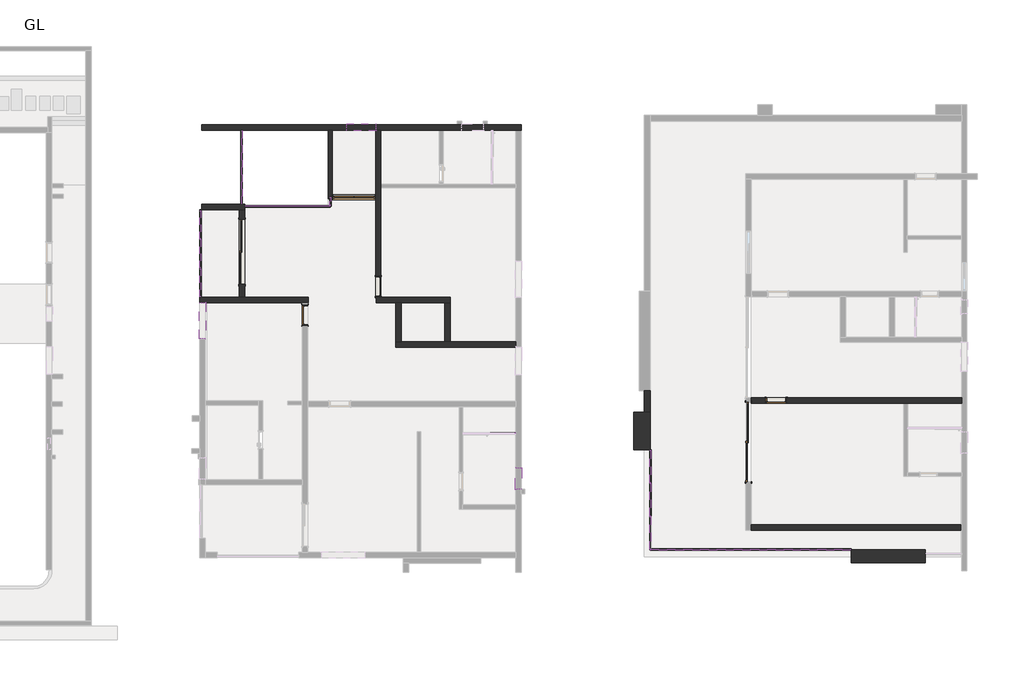
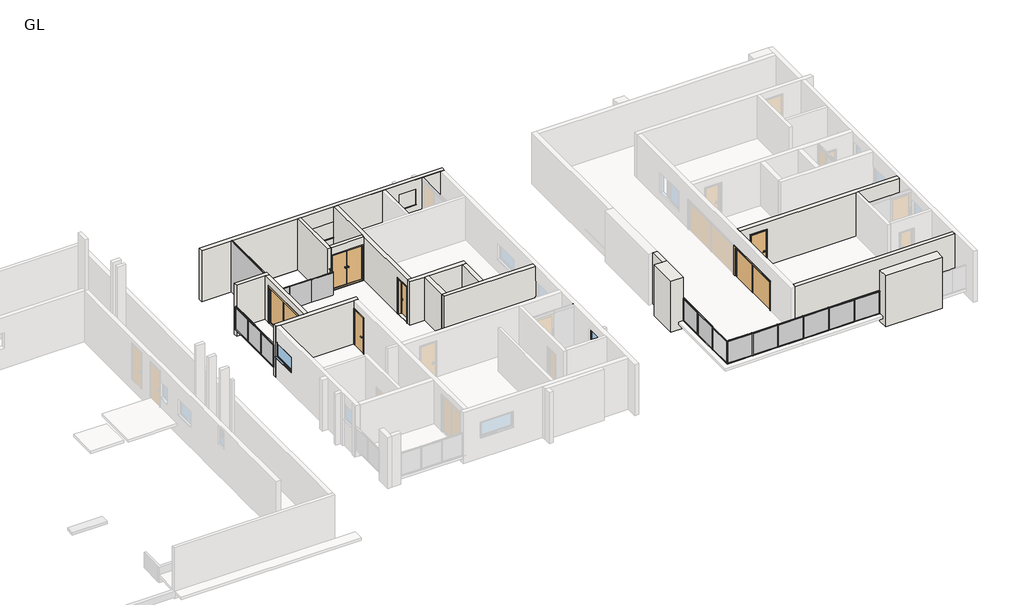
# One storey, part 3 of 6: 60 members, 17 walls, 16 plates, 6 doors, 3 windows.
"""IFC4 building model written with IfcOpenShell, lengths in millimetres."""

from ifc_helpers import new_model, si_unit, frame, origin, origin_with_axes, place, context, project, spatial, polyline, outline, extrude, faceted_brep, transform, mapped, element, save
from components import door_11_423d414f, door_9_db2a89ef, doors_extdbl_flush_1810x2110mm_0705243e, door_61435f0d, rectangular_mullion_30mm_square_7ad516a4, rectangular_mullion_30mm_square_4b249e81, rectangular_mullion_30mm_square_cc57b060, rectangular_mullion_30mm_square_bfb5791d, rectangular_mullion_30mm_square_48e0410f, rectangular_mullion_30mm_square_a54bfe06, rectangular_mullion_30mm_square_817e3251, rectangular_mullion_30mm_square_75078aee, rectangular_mullion_30mm_square_ea944ed7, rectangular_mullion_30mm_square_eb1e678b, rectangular_mullion_30mm_square_4b8855c0, rectangular_mullion_30mm_square_0acd70fe, rectangular_mullion_30mm_square_cec16e38, rectangular_mullion_30mm_square_28ebc8b3, rectangular_mullion_30mm_square_b4ecd99e, rectangular_mullion_30mm_square_04db908b, system_panel_glazed_bb4db1d5, system_panel_glazed_b6747f4f, system_panel_glazed_7e3392a4, system_panel_glazed_b055ca82, system_panel_glazed_df7e0718, system_panel_glazed_e520f566, windows_sgl_plain_3_28d0678b, windows_sgl_plain_4_aaf4c78a, windows_sgl_plain_5_79f17ecf

model = new_model("IFC4")

# Units and contexts
model_context = context("Model", 3, world=origin())
ifc_project = project(units=[si_unit("LENGTHUNIT", "METRE", prefix="MILLI")], contexts=[model_context])

# Site, building, storey
site = spatial("IfcSite", under=ifc_project)
building = spatial("IfcBuilding", under=site)
storey = spatial("IfcBuildingStorey", under=building, Name="GL", Elevation=0.0)

# Doors
placement = place(None, origin())
door_11_shape = door_11_423d414f(model_context)
element("IfcDoor", 1, ObjectType="11'", at=placement, inside=storey, context=model_context, shape_type="MappedRepresentation", body=[
    mapped(door_11_shape, transform((-5795.6337573, 13858.7592769, 0.0), x_axis=(0.0, 1.0, 0.0), y_axis=(-1.0, 0.0, 0.0), z_axis=(0.0, 0.0, 1.0))),
])
door_9_shape = door_9_db2a89ef(model_context)
element("IfcDoor", 2, ObjectType="9'", at=placement, inside=storey, context=model_context, shape_type="MappedRepresentation", body=[
    mapped(door_9_shape, transform((-27240.0290532, 21905.9424071, 449.9570313), x_axis=(0.0, 1.0, 0.0), y_axis=(-1.0, 0.0, 0.0), z_axis=(0.0, 0.0, 1.0))),
])
doors_extdbl_flush_1810x2110mm_shape = doors_extdbl_flush_1810x2110mm_0705243e(model_context)
element("IfcDoor", 3, ObjectType="Doors_ExtDbl_Flush : 1810x2110mm", at=placement, inside=storey, context=model_context, shape_type="MappedRepresentation", body=[
    mapped(doors_extdbl_flush_1810x2110mm_shape, transform((-22629.3263661, 24241.3956166, 449.9429688), x_axis=(-1.0, 0.0, 0.0), y_axis=(0.0, -1.0, 0.0), z_axis=(0.0, 0.0, 1.0))),
])
door_shape = door_61435f0d(model_context)
element("IfcDoor", 4, ObjectType="Doors_IntSgl : 2'11\"", at=placement, inside=storey, context=model_context, shape_type="MappedRepresentation", body=[
    mapped(door_shape, transform((-24702.6081987, 19226.2424071, 449.9429688), x_axis=(0.0, 1.0, 0.0), y_axis=(-1.0, 0.0, 0.0), z_axis=(0.0, 0.0, 1.0))),
])
element("IfcDoor", 5, ObjectType="Doors_IntSgl : 2'11\"", at=placement, inside=storey, context=model_context, shape_type="MappedRepresentation", body=[
    mapped(door_shape, transform((-21600.6263661, 20440.198106, 449.9429688), x_axis=(0.0, -1.0, 0.0), y_axis=(1.0, 0.0, 0.0), z_axis=(0.0, 0.0, 1.0))),
])
element("IfcDoor", 6, ObjectType="Doors_IntSgl : 2'11\"", at=placement, inside=storey, context=model_context, shape_type="MappedRepresentation", body=[
    mapped(door_shape, transform((-4754.2337573, 15621.2220058, 449.9570313), x_axis=(-1.0, 0.0, 0.0), y_axis=(0.0, -1.0, 0.0), z_axis=(0.0, 0.0, 1.0))),
])

# Members
rectangular_mullion_30mm_square_shape = rectangular_mullion_30mm_square_7ad516a4(model_context)
element("IfcMember", 7, ObjectType="Rectangular Mullion : 30mm_Square", at=placement, inside=storey, context=model_context, shape_type="MappedRepresentation", body=[
    mapped(rectangular_mullion_30mm_square_shape, transform((-24839.3272619, 23844.5206166, 449.9570313), x_axis=(-1.0, 0.0, 0.0), y_axis=(0.0, 1.0, 0.0), z_axis=(0.0, 0.0, -1.0))),
])
element("IfcMember", 8, ObjectType="Rectangular Mullion : 30mm_Square", at=placement, inside=storey, context=model_context, shape_type="MappedRepresentation", body=[
    mapped(rectangular_mullion_30mm_square_shape, transform((-26046.0281574, 23844.5206166, 449.9570313), x_axis=(-1.0, 0.0, 0.0), y_axis=(0.0, 1.0, 0.0), z_axis=(0.0, 0.0, -1.0))),
])
element("IfcMember", 9, ObjectType="Rectangular Mullion : 30mm_Square", at=placement, inside=storey, context=model_context, shape_type="MappedRepresentation", body=[
    mapped(rectangular_mullion_30mm_square_shape, transform((-29138.6790532, 22447.8090736, 449.9570313), x_axis=(0.0, -1.0, 0.0), y_axis=(-1.0, 0.0, 0.0), z_axis=(0.0, 0.0, -1.0))),
])
element("IfcMember", 10, ObjectType="Rectangular Mullion : 30mm_Square", at=placement, inside=storey, context=model_context, shape_type="MappedRepresentation", body=[
    mapped(rectangular_mullion_30mm_square_shape, transform((-29138.6790532, 21211.6757405, 449.9570313), x_axis=(0.0, -1.0, 0.0), y_axis=(-1.0, 0.0, 0.0), z_axis=(0.0, 0.0, -1.0))),
])
element("IfcMember", 11, ObjectType="Rectangular Mullion : 30mm_Square", at=placement, inside=storey, context=model_context, shape_type="MappedRepresentation", body=[
    mapped(rectangular_mullion_30mm_square_shape, transform((-10088.6061453, 12115.501348, 449.9570313), x_axis=(0.0, -1.0, 0.0), y_axis=(-1.0, 0.0, 0.0), z_axis=(0.0, 0.0, -1.0))),
])
element("IfcMember", 12, ObjectType="Rectangular Mullion : 30mm_Square", at=placement, inside=storey, context=model_context, shape_type="MappedRepresentation", body=[
    mapped(rectangular_mullion_30mm_square_shape, transform((-10088.6061453, 10704.3231184, 449.9570313), x_axis=(0.0, -1.0, 0.0), y_axis=(-1.0, 0.0, 0.0), z_axis=(0.0, 0.0, -1.0))),
])
element("IfcMember", 13, ObjectType="Rectangular Mullion : 30mm_Square", at=placement, inside=storey, context=model_context, shape_type="MappedRepresentation", body=[
    mapped(rectangular_mullion_30mm_square_shape, transform((-8671.1150001, 9293.1448884, 449.9570313), x_axis=(1.0, 0.0, 0.0), y_axis=(0.0, -1.0, 0.0), z_axis=(0.0, 0.0, -1.0))),
])
element("IfcMember", 14, ObjectType="Rectangular Mullion : 30mm_Square", at=placement, inside=storey, context=model_context, shape_type="MappedRepresentation", body=[
    mapped(rectangular_mullion_30mm_square_shape, transform((-7253.6238551, 9293.1448884, 449.9570313), x_axis=(1.0, 0.0, 0.0), y_axis=(0.0, -1.0, 0.0), z_axis=(0.0, 0.0, -1.0))),
])
element("IfcMember", 15, ObjectType="Rectangular Mullion : 30mm_Square", at=placement, inside=storey, context=model_context, shape_type="MappedRepresentation", body=[
    mapped(rectangular_mullion_30mm_square_shape, transform((-5836.1327101, 9293.1448884, 449.9570313), x_axis=(1.0, 0.0, 0.0), y_axis=(0.0, -1.0, 0.0), z_axis=(0.0, 0.0, -1.0))),
])
element("IfcMember", 16, ObjectType="Rectangular Mullion : 30mm_Square", at=placement, inside=storey, context=model_context, shape_type="MappedRepresentation", body=[
    mapped(rectangular_mullion_30mm_square_shape, transform((-4418.6415651, 9293.1448884, 449.9570313), x_axis=(1.0, 0.0, 0.0), y_axis=(0.0, -1.0, 0.0), z_axis=(0.0, 0.0, -1.0))),
])
element("IfcMember", 17, ObjectType="Rectangular Mullion : 30mm_Square", at=placement, inside=storey, context=model_context, shape_type="MappedRepresentation", body=[
    mapped(rectangular_mullion_30mm_square_shape, transform((-3001.1504201, 9293.1448884, 449.9570313), x_axis=(1.0, 0.0, 0.0), y_axis=(0.0, -1.0, 0.0), z_axis=(0.0, 0.0, -1.0))),
])
rectangular_mullion_30mm_square_2_shape = rectangular_mullion_30mm_square_4b249e81(model_context)
element("IfcMember", 18, ObjectType="Rectangular Mullion : 30mm_Square", at=placement, inside=storey, context=model_context, shape_type="MappedRepresentation", body=[
    mapped(rectangular_mullion_30mm_square_2_shape, transform((-23632.6263661, 23844.5206166, 1780.8), x_axis=(1.0, 0.0, 0.0), y_axis=(0.0, 1.0, 0.0), z_axis=(0.0, 0.0, 1.0))),
])
element("IfcMember", 19, ObjectType="Rectangular Mullion : 30mm_Square", at=placement, inside=storey, context=model_context, shape_type="MappedRepresentation", body=[
    mapped(rectangular_mullion_30mm_square_2_shape, transform((-23632.6263661, 24241.3956166, 1780.8), x_axis=(0.0, 1.0, 0.0), y_axis=(-1.0, 0.0, 0.0), z_axis=(0.0, 0.0, 1.0))),
])
element("IfcMember", 20, ObjectType="Rectangular Mullion : 30mm_Square", at=placement, inside=storey, context=model_context, shape_type="MappedRepresentation", body=[
    mapped(rectangular_mullion_30mm_square_2_shape, transform((-29138.6790532, 23683.9424071, 1780.8), x_axis=(0.0, 1.0, 0.0), y_axis=(-1.0, 0.0, 0.0), z_axis=(0.0, 0.0, 1.0))),
])
element("IfcMember", 21, ObjectType="Rectangular Mullion : 30mm_Square", at=placement, inside=storey, context=model_context, shape_type="MappedRepresentation", body=[
    mapped(rectangular_mullion_30mm_square_2_shape, transform((-10088.6061453, 13526.6795779, 1780.8), x_axis=(0.0, 1.0, 0.0), y_axis=(-1.0, 0.0, 0.0), z_axis=(0.0, 0.0, 1.0))),
])
element("IfcMember", 22, ObjectType="Rectangular Mullion : 30mm_Square", at=placement, inside=storey, context=model_context, shape_type="MappedRepresentation", body=[
    mapped(rectangular_mullion_30mm_square_2_shape, transform((-10088.6061453, 9293.1448884, 1780.8), x_axis=(-1.0, 0.0, 0.0), y_axis=(0.0, -1.0, 0.0), z_axis=(0.0, 0.0, 1.0))),
])
element("IfcMember", 23, ObjectType="Rectangular Mullion : 30mm_Square", at=placement, inside=storey, context=model_context, shape_type="MappedRepresentation", body=[
    mapped(rectangular_mullion_30mm_square_2_shape, transform((-27252.7290532, 23844.5206166, 449.9570313), x_axis=(-1.0, 0.0, 0.0), y_axis=(0.0, 1.0, 0.0), z_axis=(0.0, 0.0, -1.0))),
])
element("IfcMember", 24, ObjectType="Rectangular Mullion : 30mm_Square", at=placement, inside=storey, context=model_context, shape_type="MappedRepresentation", body=[
    mapped(rectangular_mullion_30mm_square_2_shape, transform((-23632.6263661, 23844.5206166, 449.9570313), x_axis=(0.0, -1.0, 0.0), y_axis=(-1.0, 0.0, 0.0), z_axis=(0.0, 0.0, -1.0))),
])
element("IfcMember", 25, ObjectType="Rectangular Mullion : 30mm_Square", at=placement, inside=storey, context=model_context, shape_type="MappedRepresentation", body=[
    mapped(rectangular_mullion_30mm_square_2_shape, transform((-29138.6790532, 19975.5424071, 449.9570313), x_axis=(0.0, -1.0, 0.0), y_axis=(-1.0, 0.0, 0.0), z_axis=(0.0, 0.0, -1.0))),
])
element("IfcMember", 26, ObjectType="Rectangular Mullion : 30mm_Square", at=placement, inside=storey, context=model_context, shape_type="MappedRepresentation", body=[
    mapped(rectangular_mullion_30mm_square_2_shape, transform((-10088.6061453, 9293.1448884, 449.9570313), x_axis=(0.0, -1.0, 0.0), y_axis=(-1.0, 0.0, 0.0), z_axis=(0.0, 0.0, -1.0))),
])
element("IfcMember", 27, ObjectType="Rectangular Mullion : 30mm_Square", at=placement, inside=storey, context=model_context, shape_type="MappedRepresentation", body=[
    mapped(rectangular_mullion_30mm_square_2_shape, transform((-1583.6592749, 9293.1448884, 449.9570313), x_axis=(1.0, 0.0, 0.0), y_axis=(0.0, -1.0, 0.0), z_axis=(0.0, 0.0, -1.0))),
])
rectangular_mullion_30mm_square_3_shape = rectangular_mullion_30mm_square_cc57b060(model_context)
element("IfcMember", 28, ObjectType="Rectangular Mullion : 30mm_Square", at=placement, inside=storey, context=model_context, shape_type="MappedRepresentation", body=[
    mapped(rectangular_mullion_30mm_square_3_shape, transform((-29138.6790532, 20005.5424071, 1780.8), x_axis=(0.0, 0.0, 1.0), y_axis=(-1.0, 0.0, 0.0), z_axis=(0.0, -1.0, 0.0))),
])
element("IfcMember", 29, ObjectType="Rectangular Mullion : 30mm_Square", at=placement, inside=storey, context=model_context, shape_type="MappedRepresentation", body=[
    mapped(rectangular_mullion_30mm_square_3_shape, transform((-29138.6790532, 22462.8090736, 1780.8), x_axis=(0.0, 0.0, 1.0), y_axis=(-1.0, 0.0, 0.0), z_axis=(0.0, -1.0, 0.0))),
])
element("IfcMember", 30, ObjectType="Rectangular Mullion : 30mm_Square", at=placement, inside=storey, context=model_context, shape_type="MappedRepresentation", body=[
    mapped(rectangular_mullion_30mm_square_3_shape, transform((-29138.6790532, 23653.9424071, 449.9570313), x_axis=(0.0, 0.0, -1.0), y_axis=(-1.0, 0.0, 0.0), z_axis=(0.0, 1.0, 0.0))),
])
element("IfcMember", 31, ObjectType="Rectangular Mullion : 30mm_Square", at=placement, inside=storey, context=model_context, shape_type="MappedRepresentation", body=[
    mapped(rectangular_mullion_30mm_square_3_shape, transform((-29138.6790532, 21196.6757405, 449.9570313), x_axis=(0.0, 0.0, -1.0), y_axis=(-1.0, 0.0, 0.0), z_axis=(0.0, 1.0, 0.0))),
])
rectangular_mullion_30mm_square_4_shape = rectangular_mullion_30mm_square_bfb5791d(model_context)
element("IfcMember", 32, ObjectType="Rectangular Mullion : 30mm_Square", at=placement, inside=storey, context=model_context, shape_type="MappedRepresentation", body=[
    mapped(rectangular_mullion_30mm_square_4_shape, transform((-29138.6790532, 22432.8090736, 449.9570313), x_axis=(0.0, 0.0, -1.0), y_axis=(-1.0, 0.0, 0.0), z_axis=(0.0, 1.0, 0.0))),
])
element("IfcMember", 33, ObjectType="Rectangular Mullion : 30mm_Square", at=placement, inside=storey, context=model_context, shape_type="MappedRepresentation", body=[
    mapped(rectangular_mullion_30mm_square_4_shape, transform((-29138.6790532, 21226.6757405, 1780.8), x_axis=(0.0, 0.0, 1.0), y_axis=(-1.0, 0.0, 0.0), z_axis=(0.0, -1.0, 0.0))),
])
rectangular_mullion_30mm_square_5_shape = rectangular_mullion_30mm_square_48e0410f(model_context)
element("IfcMember", 34, ObjectType="Rectangular Mullion : 30mm_Square", at=placement, inside=storey, context=model_context, shape_type="MappedRepresentation", body=[
    mapped(rectangular_mullion_30mm_square_5_shape, transform((-10088.6061453, 9323.1448884, 1780.8), x_axis=(0.0, 0.0, 1.0), y_axis=(-1.0, 0.0, 0.0), z_axis=(0.0, -1.0, 0.0))),
])
element("IfcMember", 35, ObjectType="Rectangular Mullion : 30mm_Square", at=placement, inside=storey, context=model_context, shape_type="MappedRepresentation", body=[
    mapped(rectangular_mullion_30mm_square_5_shape, transform((-10088.6061453, 12130.501348, 1780.8), x_axis=(0.0, 0.0, 1.0), y_axis=(-1.0, 0.0, 0.0), z_axis=(0.0, -1.0, 0.0))),
])
element("IfcMember", 36, ObjectType="Rectangular Mullion : 30mm_Square", at=placement, inside=storey, context=model_context, shape_type="MappedRepresentation", body=[
    mapped(rectangular_mullion_30mm_square_5_shape, transform((-10088.6061453, 13496.6795779, 449.9570313), x_axis=(0.0, 0.0, -1.0), y_axis=(-1.0, 0.0, 0.0), z_axis=(0.0, 1.0, 0.0))),
])
element("IfcMember", 37, ObjectType="Rectangular Mullion : 30mm_Square", at=placement, inside=storey, context=model_context, shape_type="MappedRepresentation", body=[
    mapped(rectangular_mullion_30mm_square_5_shape, transform((-10088.6061453, 10689.3231184, 449.9570313), x_axis=(0.0, 0.0, -1.0), y_axis=(-1.0, 0.0, 0.0), z_axis=(0.0, 1.0, 0.0))),
])
rectangular_mullion_30mm_square_6_shape = rectangular_mullion_30mm_square_a54bfe06(model_context)
element("IfcMember", 38, ObjectType="Rectangular Mullion : 30mm_Square", at=placement, inside=storey, context=model_context, shape_type="MappedRepresentation", body=[
    mapped(rectangular_mullion_30mm_square_6_shape, transform((-10088.6061453, 12100.501348, 449.9570313), x_axis=(0.0, 0.0, -1.0), y_axis=(-1.0, 0.0, 0.0), z_axis=(0.0, 1.0, 0.0))),
])
element("IfcMember", 39, ObjectType="Rectangular Mullion : 30mm_Square", at=placement, inside=storey, context=model_context, shape_type="MappedRepresentation", body=[
    mapped(rectangular_mullion_30mm_square_6_shape, transform((-10088.6061453, 10719.3231184, 1780.8), x_axis=(0.0, 0.0, 1.0), y_axis=(-1.0, 0.0, 0.0), z_axis=(0.0, -1.0, 0.0))),
])
rectangular_mullion_30mm_square_7_shape = rectangular_mullion_30mm_square_817e3251(model_context)
element("IfcMember", 40, ObjectType="Rectangular Mullion : 30mm_Square", at=placement, inside=storey, context=model_context, shape_type="MappedRepresentation", body=[
    mapped(rectangular_mullion_30mm_square_7_shape, transform((-1613.6592749, 9293.1448884, 1780.8), x_axis=(0.0, 0.0, 1.0), y_axis=(0.0, -1.0, 0.0), z_axis=(1.0, 0.0, 0.0))),
])
element("IfcMember", 41, ObjectType="Rectangular Mullion : 30mm_Square", at=placement, inside=storey, context=model_context, shape_type="MappedRepresentation", body=[
    mapped(rectangular_mullion_30mm_square_7_shape, transform((-8686.1150001, 9293.1448884, 1780.8), x_axis=(0.0, 0.0, 1.0), y_axis=(0.0, -1.0, 0.0), z_axis=(1.0, 0.0, 0.0))),
])
element("IfcMember", 42, ObjectType="Rectangular Mullion : 30mm_Square", at=placement, inside=storey, context=model_context, shape_type="MappedRepresentation", body=[
    mapped(rectangular_mullion_30mm_square_7_shape, transform((-10058.6061453, 9293.1448884, 449.9570313), x_axis=(0.0, 0.0, -1.0), y_axis=(0.0, -1.0, 0.0), z_axis=(-1.0, 0.0, 0.0))),
])
element("IfcMember", 43, ObjectType="Rectangular Mullion : 30mm_Square", at=placement, inside=storey, context=model_context, shape_type="MappedRepresentation", body=[
    mapped(rectangular_mullion_30mm_square_7_shape, transform((-2986.1504201, 9293.1448884, 449.9570313), x_axis=(0.0, 0.0, -1.0), y_axis=(0.0, -1.0, 0.0), z_axis=(-1.0, 0.0, 0.0))),
])
rectangular_mullion_30mm_square_8_shape = rectangular_mullion_30mm_square_75078aee(model_context)
element("IfcMember", 44, ObjectType="Rectangular Mullion : 30mm_Square", at=placement, inside=storey, context=model_context, shape_type="MappedRepresentation", body=[
    mapped(rectangular_mullion_30mm_square_8_shape, transform((-8656.1150001, 9293.1448884, 449.9570313), x_axis=(0.0, 0.0, -1.0), y_axis=(0.0, -1.0, 0.0), z_axis=(-1.0, 0.0, 0.0))),
])
element("IfcMember", 45, ObjectType="Rectangular Mullion : 30mm_Square", at=placement, inside=storey, context=model_context, shape_type="MappedRepresentation", body=[
    mapped(rectangular_mullion_30mm_square_8_shape, transform((-7238.6238551, 9293.1448884, 449.9570313), x_axis=(0.0, 0.0, -1.0), y_axis=(0.0, -1.0, 0.0), z_axis=(-1.0, 0.0, 0.0))),
])
element("IfcMember", 46, ObjectType="Rectangular Mullion : 30mm_Square", at=placement, inside=storey, context=model_context, shape_type="MappedRepresentation", body=[
    mapped(rectangular_mullion_30mm_square_8_shape, transform((-5821.1327101, 9293.1448884, 449.9570313), x_axis=(0.0, 0.0, -1.0), y_axis=(0.0, -1.0, 0.0), z_axis=(-1.0, 0.0, 0.0))),
])
element("IfcMember", 47, ObjectType="Rectangular Mullion : 30mm_Square", at=placement, inside=storey, context=model_context, shape_type="MappedRepresentation", body=[
    mapped(rectangular_mullion_30mm_square_8_shape, transform((-4403.6415651, 9293.1448884, 449.9570313), x_axis=(0.0, 0.0, -1.0), y_axis=(0.0, -1.0, 0.0), z_axis=(-1.0, 0.0, 0.0))),
])
element("IfcMember", 48, ObjectType="Rectangular Mullion : 30mm_Square", at=placement, inside=storey, context=model_context, shape_type="MappedRepresentation", body=[
    mapped(rectangular_mullion_30mm_square_8_shape, transform((-7268.6238551, 9293.1448884, 1780.8), x_axis=(0.0, 0.0, 1.0), y_axis=(0.0, -1.0, 0.0), z_axis=(1.0, 0.0, 0.0))),
])
element("IfcMember", 49, ObjectType="Rectangular Mullion : 30mm_Square", at=placement, inside=storey, context=model_context, shape_type="MappedRepresentation", body=[
    mapped(rectangular_mullion_30mm_square_8_shape, transform((-5851.1327101, 9293.1448884, 1780.8), x_axis=(0.0, 0.0, 1.0), y_axis=(0.0, -1.0, 0.0), z_axis=(1.0, 0.0, 0.0))),
])
element("IfcMember", 50, ObjectType="Rectangular Mullion : 30mm_Square", at=placement, inside=storey, context=model_context, shape_type="MappedRepresentation", body=[
    mapped(rectangular_mullion_30mm_square_8_shape, transform((-4433.6415651, 9293.1448884, 1780.8), x_axis=(0.0, 0.0, 1.0), y_axis=(0.0, -1.0, 0.0), z_axis=(1.0, 0.0, 0.0))),
])
element("IfcMember", 51, ObjectType="Rectangular Mullion : 30mm_Square", at=placement, inside=storey, context=model_context, shape_type="MappedRepresentation", body=[
    mapped(rectangular_mullion_30mm_square_8_shape, transform((-3016.1504201, 9293.1448884, 1780.8), x_axis=(0.0, 0.0, 1.0), y_axis=(0.0, -1.0, 0.0), z_axis=(1.0, 0.0, 0.0))),
])
rectangular_mullion_30mm_square_9_shape = rectangular_mullion_30mm_square_ea944ed7(model_context)
element("IfcMember", 52, ObjectType="Rectangular Mullion : 30mm_Square", at=placement, inside=storey, context=model_context, shape_type="MappedRepresentation", body=[
    mapped(rectangular_mullion_30mm_square_9_shape, transform((-27222.7290532, 23844.5206166, 1780.8), x_axis=(0.0, 0.0, 1.0), y_axis=(0.0, 1.0, 0.0), z_axis=(-1.0, 0.0, 0.0))),
])
element("IfcMember", 53, ObjectType="Rectangular Mullion : 30mm_Square", at=placement, inside=storey, context=model_context, shape_type="MappedRepresentation", body=[
    mapped(rectangular_mullion_30mm_square_9_shape, transform((-24824.3272619, 23844.5206166, 1780.8), x_axis=(0.0, 0.0, 1.0), y_axis=(0.0, 1.0, 0.0), z_axis=(-1.0, 0.0, 0.0))),
])
element("IfcMember", 54, ObjectType="Rectangular Mullion : 30mm_Square", at=placement, inside=storey, context=model_context, shape_type="MappedRepresentation", body=[
    mapped(rectangular_mullion_30mm_square_9_shape, transform((-23662.6263661, 23844.5206166, 449.9570313), x_axis=(0.0, 0.0, -1.0), y_axis=(0.0, 1.0, 0.0), z_axis=(1.0, 0.0, 0.0))),
])
element("IfcMember", 55, ObjectType="Rectangular Mullion : 30mm_Square", at=placement, inside=storey, context=model_context, shape_type="MappedRepresentation", body=[
    mapped(rectangular_mullion_30mm_square_9_shape, transform((-26061.0281574, 23844.5206166, 449.9570313), x_axis=(0.0, 0.0, -1.0), y_axis=(0.0, 1.0, 0.0), z_axis=(1.0, 0.0, 0.0))),
])
rectangular_mullion_30mm_square_10_shape = rectangular_mullion_30mm_square_eb1e678b(model_context)
element("IfcMember", 56, ObjectType="Rectangular Mullion : 30mm_Square", at=placement, inside=storey, context=model_context, shape_type="MappedRepresentation", body=[
    mapped(rectangular_mullion_30mm_square_10_shape, transform((-24854.3272619, 23844.5206166, 449.9570313), x_axis=(0.0, 0.0, -1.0), y_axis=(0.0, 1.0, 0.0), z_axis=(1.0, 0.0, 0.0))),
])
element("IfcMember", 57, ObjectType="Rectangular Mullion : 30mm_Square", at=placement, inside=storey, context=model_context, shape_type="MappedRepresentation", body=[
    mapped(rectangular_mullion_30mm_square_10_shape, transform((-26031.0281574, 23844.5206166, 1780.8), x_axis=(0.0, 0.0, 1.0), y_axis=(0.0, 1.0, 0.0), z_axis=(-1.0, 0.0, 0.0))),
])
rectangular_mullion_30mm_square_11_shape = rectangular_mullion_30mm_square_4b8855c0(model_context)
element("IfcMember", 58, ObjectType="Rectangular Mullion : 30mm_Square", at=placement, inside=storey, context=model_context, shape_type="MappedRepresentation", body=[
    mapped(rectangular_mullion_30mm_square_11_shape, transform((-27367.0290532, 27029.0409184, 3000.0), x_axis=(0.0, 0.0, 1.0), y_axis=(1.0, 0.0, 0.0), z_axis=(0.0, 1.0, 0.0))),
])
element("IfcMember", 59, ObjectType="Rectangular Mullion : 30mm_Square", at=placement, inside=storey, context=model_context, shape_type="MappedRepresentation", body=[
    mapped(rectangular_mullion_30mm_square_11_shape, transform((-27367.0290532, 23942.5424071, 0.0), x_axis=(0.0, 0.0, -1.0), y_axis=(1.0, 0.0, 0.0), z_axis=(0.0, -1.0, 0.0))),
])
rectangular_mullion_30mm_square_12_shape = rectangular_mullion_30mm_square_0acd70fe(model_context)
element("IfcMember", 60, ObjectType="Rectangular Mullion : 30mm_Square", at=placement, inside=storey, context=model_context, shape_type="MappedRepresentation", body=[
    mapped(rectangular_mullion_30mm_square_12_shape, transform((-27367.0290532, 23912.5424071, 3000.0), x_axis=(0.0, -1.0, 0.0), y_axis=(1.0, 0.0, 0.0), z_axis=(0.0, 0.0, 1.0))),
])
element("IfcMember", 61, ObjectType="Rectangular Mullion : 30mm_Square", at=placement, inside=storey, context=model_context, shape_type="MappedRepresentation", body=[
    mapped(rectangular_mullion_30mm_square_12_shape, transform((-27367.0290532, 27059.0409184, 0.0), x_axis=(0.0, 1.0, 0.0), y_axis=(1.0, 0.0, 0.0), z_axis=(0.0, 0.0, -1.0))),
])
rectangular_mullion_30mm_square_13_shape = rectangular_mullion_30mm_square_cec16e38(model_context)
element("IfcMember", 62, ObjectType="Rectangular Mullion : 30mm_Square", at=placement, inside=storey, context=model_context, shape_type="MappedRepresentation", body=[
    mapped(rectangular_mullion_30mm_square_13_shape, transform((-23632.6263661, 23874.5206166, 1780.8), x_axis=(0.0, 0.0, 1.0), y_axis=(-1.0, 0.0, 0.0), z_axis=(0.0, -1.0, 0.0))),
])
element("IfcMember", 63, ObjectType="Rectangular Mullion : 30mm_Square", at=placement, inside=storey, context=model_context, shape_type="MappedRepresentation", body=[
    mapped(rectangular_mullion_30mm_square_13_shape, transform((-23632.6263661, 24211.3956166, 449.9570313), x_axis=(0.0, 0.0, -1.0), y_axis=(-1.0, 0.0, 0.0), z_axis=(0.0, 1.0, 0.0))),
])
rectangular_mullion_30mm_square_14_shape = rectangular_mullion_30mm_square_28ebc8b3(model_context)
element("IfcMember", 64, ObjectType="Rectangular Mullion : 30mm_Square", at=placement, inside=storey, context=model_context, shape_type="MappedRepresentation", body=[
    mapped(rectangular_mullion_30mm_square_14_shape, transform((-15791.6562878, 14231.6822323, 3000.0), x_axis=(1.0, 0.0, 0.0), y_axis=(0.0, 1.0, 0.0), z_axis=(0.0, 0.0, 1.0))),
])
rectangular_mullion_30mm_square_15_shape = rectangular_mullion_30mm_square_b4ecd99e(model_context)
element("IfcMember", 65, ObjectType="Rectangular Mullion : 30mm_Square", at=placement, inside=storey, context=model_context, shape_type="MappedRepresentation", body=[
    mapped(rectangular_mullion_30mm_square_15_shape, transform((-15791.6562878, 14231.6822323, 2849.9570312), x_axis=(1.0, 0.0, 0.0), y_axis=(0.0, 1.0, 0.0), z_axis=(0.0, 0.0, 1.0))),
])
rectangular_mullion_30mm_square_16_shape = rectangular_mullion_30mm_square_04db908b(model_context)
element("IfcMember", 66, ObjectType="Rectangular Mullion : 30mm_Square", at=placement, inside=storey, context=model_context, shape_type="MappedRepresentation", body=[
    mapped(rectangular_mullion_30mm_square_16_shape, transform((-15821.6562878, 14231.6822323, 449.9570313), x_axis=(0.0, 0.0, -1.0), y_axis=(0.0, 1.0, 0.0), z_axis=(1.0, 0.0, 0.0))),
])

# Plates
system_panel_glazed_shape = system_panel_glazed_bb4db1d5(model_context)
element("IfcPlate", 67, ObjectType="System Panel : Glazed", at=placement, inside=storey, context=model_context, shape_type="MappedRepresentation", body=[
    mapped(system_panel_glazed_shape, transform((-29138.6790532, 23065.8757403, 449.9570313), x_axis=(0.0, -1.0, 0.0), y_axis=(1.0, 0.0, 0.0), z_axis=(0.0, 0.0, 1.0))),
])
element("IfcPlate", 68, ObjectType="System Panel : Glazed", at=placement, inside=storey, context=model_context, shape_type="MappedRepresentation", body=[
    mapped(system_panel_glazed_shape, transform((-29138.6790532, 21829.7424071, 449.9570313), x_axis=(0.0, -1.0, 0.0), y_axis=(1.0, 0.0, 0.0), z_axis=(0.0, 0.0, 1.0))),
])
element("IfcPlate", 69, ObjectType="System Panel : Glazed", at=placement, inside=storey, context=model_context, shape_type="MappedRepresentation", body=[
    mapped(system_panel_glazed_shape, transform((-29138.6790532, 20593.6090738, 449.9570313), x_axis=(0.0, -1.0, 0.0), y_axis=(1.0, 0.0, 0.0), z_axis=(0.0, 0.0, 1.0))),
])
system_panel_glazed_2_shape = system_panel_glazed_b6747f4f(model_context)
element("IfcPlate", 70, ObjectType="System Panel : Glazed", at=placement, inside=storey, context=model_context, shape_type="MappedRepresentation", body=[
    mapped(system_panel_glazed_2_shape, transform((-10088.6061453, 12821.0904629, 449.9570313), x_axis=(0.0, -1.0, 0.0), y_axis=(1.0, 0.0, 0.0), z_axis=(0.0, 0.0, 1.0))),
])
element("IfcPlate", 71, ObjectType="System Panel : Glazed", at=placement, inside=storey, context=model_context, shape_type="MappedRepresentation", body=[
    mapped(system_panel_glazed_2_shape, transform((-10088.6061453, 11409.9122332, 449.9570313), x_axis=(0.0, -1.0, 0.0), y_axis=(1.0, 0.0, 0.0), z_axis=(0.0, 0.0, 1.0))),
])
system_panel_glazed_3_shape = system_panel_glazed_7e3392a4(model_context)
element("IfcPlate", 72, ObjectType="System Panel : Glazed", at=placement, inside=storey, context=model_context, shape_type="MappedRepresentation", body=[
    mapped(system_panel_glazed_3_shape, transform((-9379.8605727, 9293.1448884, 449.9570313), x_axis=(1.0, 0.0, 0.0), y_axis=(0.0, 1.0, 0.0), z_axis=(0.0, 0.0, 1.0))),
])
element("IfcPlate", 73, ObjectType="System Panel : Glazed", at=placement, inside=storey, context=model_context, shape_type="MappedRepresentation", body=[
    mapped(system_panel_glazed_3_shape, transform((-7962.3694276, 9293.1448884, 449.9570313), x_axis=(1.0, 0.0, 0.0), y_axis=(0.0, 1.0, 0.0), z_axis=(0.0, 0.0, 1.0))),
])
element("IfcPlate", 74, ObjectType="System Panel : Glazed", at=placement, inside=storey, context=model_context, shape_type="MappedRepresentation", body=[
    mapped(system_panel_glazed_3_shape, transform((-6544.8782826, 9293.1448884, 449.9570313), x_axis=(1.0, 0.0, 0.0), y_axis=(0.0, 1.0, 0.0), z_axis=(0.0, 0.0, 1.0))),
])
element("IfcPlate", 75, ObjectType="System Panel : Glazed", at=placement, inside=storey, context=model_context, shape_type="MappedRepresentation", body=[
    mapped(system_panel_glazed_3_shape, transform((-5127.3871376, 9293.1448884, 449.9570313), x_axis=(1.0, 0.0, 0.0), y_axis=(0.0, 1.0, 0.0), z_axis=(0.0, 0.0, 1.0))),
])
element("IfcPlate", 76, ObjectType="System Panel : Glazed", at=placement, inside=storey, context=model_context, shape_type="MappedRepresentation", body=[
    mapped(system_panel_glazed_3_shape, transform((-3709.8959926, 9293.1448884, 449.9570313), x_axis=(1.0, 0.0, 0.0), y_axis=(0.0, 1.0, 0.0), z_axis=(0.0, 0.0, 1.0))),
])
element("IfcPlate", 77, ObjectType="System Panel : Glazed", at=placement, inside=storey, context=model_context, shape_type="MappedRepresentation", body=[
    mapped(system_panel_glazed_3_shape, transform((-2292.4048475, 9293.1448884, 449.9570313), x_axis=(1.0, 0.0, 0.0), y_axis=(0.0, 1.0, 0.0), z_axis=(0.0, 0.0, 1.0))),
])
system_panel_glazed_4_shape = system_panel_glazed_b055ca82(model_context)
element("IfcPlate", 78, ObjectType="System Panel : Glazed", at=placement, inside=storey, context=model_context, shape_type="MappedRepresentation", body=[
    mapped(system_panel_glazed_4_shape, transform((-24235.976814, 23844.5206166, 449.9570313), x_axis=(-1.0, 0.0, 0.0), y_axis=(0.0, -1.0, 0.0), z_axis=(0.0, 0.0, 1.0))),
])
element("IfcPlate", 79, ObjectType="System Panel : Glazed", at=placement, inside=storey, context=model_context, shape_type="MappedRepresentation", body=[
    mapped(system_panel_glazed_4_shape, transform((-25442.6777096, 23844.5206166, 449.9570313), x_axis=(-1.0, 0.0, 0.0), y_axis=(0.0, -1.0, 0.0), z_axis=(0.0, 0.0, 1.0))),
])
element("IfcPlate", 80, ObjectType="System Panel : Glazed", at=placement, inside=storey, context=model_context, shape_type="MappedRepresentation", body=[
    mapped(system_panel_glazed_4_shape, transform((-26649.3786053, 23844.5206166, 449.9570313), x_axis=(-1.0, 0.0, 0.0), y_axis=(0.0, -1.0, 0.0), z_axis=(0.0, 0.0, 1.0))),
])
system_panel_glazed_5_shape = system_panel_glazed_df7e0718(model_context)
element("IfcPlate", 81, ObjectType="System Panel : Glazed", at=placement, inside=storey, context=model_context, shape_type="MappedRepresentation", body=[
    mapped(system_panel_glazed_5_shape, transform((-27367.0290532, 25485.7916627, 0.0), x_axis=(0.0, 1.0, 0.0), y_axis=(-1.0, 0.0, 0.0), z_axis=(0.0, 0.0, 1.0))),
])
system_panel_glazed_6_shape = system_panel_glazed_e520f566(model_context)
element("IfcPlate", 82, ObjectType="System Panel : Glazed", at=placement, inside=storey, context=model_context, shape_type="MappedRepresentation", body=[
    mapped(system_panel_glazed_6_shape, transform((-23632.6263661, 24042.9581166, 449.9570313), x_axis=(0.0, -1.0, 0.0), y_axis=(1.0, 0.0, 0.0), z_axis=(0.0, 0.0, 1.0))),
])

# Walls
element("IfcWall", 83, ObjectType="1'10\"", at=placement, inside=storey, context=model_context, shape_type="SweptSolid", body=[
    extrude(outline(polyline([(-1583.6592749, 9293.1448884), (1565.9407251, 9293.1448884), (1565.9407251, 8734.3448884), (-1583.6592749, 8734.3448884), (-1583.6592749, 9293.1448884)])), origin_with_axes(), (0.0, 0.0, 1.0), 3000.0),
])
element("IfcWall", 84, ObjectType="10\"", at=placement, inside=storey, context=model_context, shape_type="SweptSolid", body=[
    extrude(outline(polyline([(-10088.6061453, 16028.5795779), (-10088.6061453, 15114.1795779), (-10342.6061453, 15114.1795779), (-10342.6061453, 16028.5795779), (-10088.6061453, 16028.5795779)])), origin_with_axes(), (0.0, 0.0, 1.0), 3000.0),
])
element("IfcWall", 85, ObjectType="2'3\"", at=placement, inside=storey, context=model_context, shape_type="Brep", body=[
    faceted_brep([(-10088.6061453, 13526.6795779, 0.0), (-10088.6061453, 15114.1795779, 0.0), (-10088.6061453, 15114.1795779, 3000.0), (-10088.6061453, 13526.6795779, 3000.0), (-10774.4061453, 13526.6795779, 0.0), (-10774.4061453, 13526.6795779, 3000.0), (-10774.4061453, 15114.1795779, 3000.0), (-10774.4061453, 15114.1795779, 0.0), (-10342.6061453, 15114.1795779, 0.0), (-10342.6061453, 15114.1795779, 3000.0)], [[[0, 1, 2, 3]], [[4, 5, 6, 7]], [[1, 0, 4, 7, 8]], [[2, 1, 8, 7, 6, 9]], [[3, 2, 9, 6, 5]], [[0, 3, 5, 4]]]),
])
element("IfcWall", 86, ObjectType="7\" WALL", at=placement, inside=storey, context=model_context, shape_type="Brep", body=[
    faceted_brep([(-23721.5263661, 27048.0956166, 0.0), (-23721.5263661, 24152.4956166, 0.0), (-23721.5263661, 24152.4956166, 3000.0), (-23721.5263661, 27048.0956166, 3000.0), (-23543.7263661, 27048.0956166, 0.0), (-23543.7263661, 27048.0956166, 3000.0), (-23543.7263661, 24330.2956166, 3000.0), (-23543.7263661, 24152.4956166, 3000.0), (-23543.7263661, 24152.4956166, 0.0), (-23543.7263661, 24330.2956166, 0.0)], [[[0, 1, 2, 3]], [[4, 5, 6, 7, 8, 9]], [[1, 0, 4, 9, 8]], [[3, 2, 7, 6, 5]], [[0, 3, 5, 4]], [[2, 1, 8, 7]]]),
])
element("IfcWall", 87, ObjectType="7\" WALL", at=placement, inside=storey, context=model_context, shape_type="SweptSolid", body=[
    extrude(outline(polyline([(0.0, -23543.7263661), (0.0, -21714.9263661), (3000.0, -21714.9263661), (3000.0, -23543.7263661), (0.0, -23543.7263661)]), holes=[polyline([(2559.9429688, -21724.3263661), (449.9429688, -21724.3263661), (449.9429688, -23534.3263661), (2559.9429688, -23534.3263661), (2559.9429688, -21724.3263661)])]), frame((0.0, 24152.4956166, 0.0), z_axis=(0.0, 1.0, 0.0), x_axis=(0.0, 0.0, 1.0)), (0.0, 0.0, 1.0), 177.8),
])
element("IfcWall", 88, ObjectType="9\" INNER WALL", at=placement, inside=storey, context=model_context, shape_type="Brep", body=[
    faceted_brep([(-15556.8464918, 27287.6409184, 0.0), (-16977.5266085, 27287.6409184, 0.0), (-17155.3266085, 27287.6409184, 0.0), (-18069.7266085, 27287.6409184, 0.0), (-18247.5266085, 27287.6409184, 0.0), (-29069.6464918, 27287.6409184, 0.0), (-29069.6464918, 27287.6409184, 3000.0), (-18247.5266085, 27287.6409184, 3000.0), (-18069.7266085, 27287.6409184, 3000.0), (-17155.3266085, 27287.6409184, 3000.0), (-16977.5266085, 27287.6409184, 3000.0), (-15556.8464918, 27287.6409184, 3000.0), (-15556.8464918, 27059.0409184, 0.0), (-15556.8464918, 27059.0409184, 3000.0), (-15785.4464918, 27059.0409184, 3000.0), (-29069.6464918, 27059.0409184, 3000.0), (-29069.6464918, 27059.0409184, 0.0), (-15785.4464918, 27059.0409184, 0.0)], [[[0, 1, 2, 3, 4, 5, 6, 7, 8, 9, 10, 11]], [[12, 13, 14, 15, 16, 17]], [[5, 4, 3, 2, 1, 0, 12, 17, 16]], [[6, 5, 16, 15]], [[11, 10, 9, 8, 7, 6, 15, 14, 13]], [[0, 11, 13, 12]]]),
])
element("IfcWall", 89, ObjectType="9\" INNER WALL", at=placement, inside=storey, context=model_context, shape_type="Brep", body=[
    faceted_brep([(-29068.8290532, 23683.9424071, 0.0), (-27481.3290532, 23683.9424071, 0.0), (-27252.7290532, 23683.9424071, 0.0), (-27252.7290532, 23683.9424071, 3000.0), (-27481.3290532, 23683.9424071, 3000.0), (-29068.8290532, 23683.9424071, 3000.0), (-29068.8290532, 23912.5424071, 0.0), (-29068.8290532, 23912.5424071, 3000.0), (-27252.7290532, 23912.5424071, 3000.0), (-27252.7290532, 23912.5424071, 0.0)], [[[0, 1, 2, 3, 4, 5]], [[6, 7, 8, 9]], [[2, 1, 0, 6, 9]], [[5, 4, 3, 8, 7]], [[0, 5, 7, 6]], [[3, 2, 9, 8]]]),
])
element("IfcWall", 90, ObjectType="9\" INNER WALL", at=placement, inside=storey, context=model_context, shape_type="SweptSolid", body=[
    extrude(outline(polyline([(23683.9424071, 0.0), (19975.5424071, 0.0), (19975.5424071, 3000.0), (23683.9424071, 3000.0), (23683.9424071, 0.0)]), holes=[polyline([(20534.3424071, 2583.9570312), (20534.3424071, 449.9570313), (23277.5424071, 449.9570313), (23277.5424071, 2583.9570312), (20534.3424071, 2583.9570312)])]), frame((-27481.3290532, 0.0, 0.0), z_axis=(1.0, 0.0, 0.0), x_axis=(0.0, 1.0, 0.0)), (0.0, 0.0, 1.0), 228.6),
])
element("IfcWall", 91, ObjectType="9\" INNER WALL", at=placement, inside=storey, context=model_context, shape_type="Brep", body=[
    faceted_brep([(-29151.3790532, 19746.9424071, 0.0), (-28922.7790532, 19746.9424071, 0.0), (-24816.9081987, 19746.9424071, 0.0), (-24588.3081987, 19746.9424071, 0.0), (-24560.3290532, 19746.9424071, 0.0), (-24560.3290532, 19746.9424071, 3000.0), (-24588.3081987, 19746.9424071, 3000.0), (-24816.9081987, 19746.9424071, 3000.0), (-28922.7790532, 19746.9424071, 3000.0), (-29151.3790532, 19746.9424071, 3000.0), (-29151.3790532, 19975.5424071, 0.0), (-29151.3790532, 19975.5424071, 3000.0), (-27481.3290532, 19975.5424071, 3000.0), (-27252.7290532, 19975.5424071, 3000.0), (-24560.3290532, 19975.5424071, 3000.0), (-24560.3290532, 19975.5424071, 0.0), (-27252.7290532, 19975.5424071, 0.0), (-27481.3290532, 19975.5424071, 0.0)], [[[0, 1, 2, 3, 4, 5, 6, 7, 8, 9]], [[10, 11, 12, 13, 14, 15, 16, 17]], [[4, 3, 2, 1, 0, 10, 17, 16, 15]], [[5, 4, 15, 14]], [[9, 8, 7, 6, 5, 14, 13, 12, 11]], [[0, 9, 11, 10]]]),
])
element("IfcWall", 92, ObjectType="9\" INNER WALL", at=placement, inside=storey, context=model_context, shape_type="Brep", body=[
    faceted_brep([(-29067.9266085, 27056.898106, 0.0), (-21714.9263661, 27056.898106, 0.0), (-21486.3263661, 27056.898106, 0.0), (-19009.5266085, 27056.898106, 0.0), (-18857.1266085, 27056.898106, 0.0), (-15556.8464918, 27056.898106, 0.0), (-15556.8464918, 27056.898106, 3000.0), (-18857.1266085, 27056.898106, 3000.0), (-19009.5266085, 27056.898106, 3000.0), (-21486.3263661, 27056.898106, 3000.0), (-21714.9263661, 27056.898106, 3000.0), (-29067.9266085, 27056.898106, 3000.0), (-22934.1263661, 27056.898106, 2110.0), (-21714.9263661, 27056.898106, 2110.0), (-21714.9263661, 27056.898106, 1200.0), (-22934.1263661, 27056.898106, 1200.0), (-18069.7266085, 27056.898106, 2434.0), (-17155.3266085, 27056.898106, 2434.0), (-17155.3266085, 27056.898106, 1524.0), (-18069.7266085, 27056.898106, 1524.0), (-29067.9266085, 27285.498106, 0.0), (-29067.9266085, 27285.498106, 3000.0), (-15556.8464918, 27285.498106, 3000.0), (-15556.8464918, 27285.498106, 0.0), (-22934.1263661, 27285.498106, 2110.0), (-22934.1263661, 27285.498106, 1200.0), (-21714.9263661, 27285.498106, 1200.0), (-21714.9263661, 27285.498106, 2110.0), (-18069.7266085, 27285.498106, 2434.0), (-18069.7266085, 27285.498106, 1524.0), (-17155.3266085, 27285.498106, 1524.0), (-17155.3266085, 27285.498106, 2434.0)], [[[0, 1, 2, 3, 4, 5, 6, 7, 8, 9, 10, 11], [12, 13, 14, 15], [16, 17, 18, 19]], [[20, 21, 22, 23], [24, 25, 26, 27], [28, 29, 30, 31]], [[5, 4, 3, 2, 1, 0, 20, 23]], [[11, 10, 9, 8, 7, 6, 22, 21]], [[0, 11, 21, 20]], [[6, 5, 23, 22]], [[25, 24, 12, 15]], [[26, 25, 15, 14]], [[27, 26, 14, 13]], [[24, 27, 13, 12]], [[29, 28, 16, 19]], [[30, 29, 19, 18]], [[31, 30, 18, 17]], [[28, 31, 17, 16]]]),
])
element("IfcWall", 93, ObjectType="9\" INNER WALL", at=placement, inside=storey, context=model_context, shape_type="Brep", body=[
    faceted_brep([(-21714.9263661, 20884.698106, 2559.9429688), (-21714.9263661, 19995.698106, 2559.9429688), (-21714.9263661, 19995.698106, 3000.0), (-21714.9263661, 24152.4956166, 3000.0), (-21714.9263661, 24330.2956166, 3000.0), (-21714.9263661, 27056.898106, 3000.0), (-21714.9263661, 27056.898106, 0.0), (-21714.9263661, 24330.2956166, 0.0), (-21714.9263661, 24152.4956166, 0.0), (-21714.9263661, 19995.698106, 0.0), (-21714.9263661, 19995.698106, 449.9429688), (-21714.9263661, 20884.698106, 449.9429688), (-21486.3263661, 19995.698106, 3000.0), (-21486.3263661, 19995.698106, 2559.9429688), (-21486.3263661, 20884.698106, 2559.9429688), (-21486.3263661, 20884.698106, 449.9429688), (-21486.3263661, 19995.698106, 449.9429688), (-21486.3263661, 19995.698106, 0.0), (-21486.3263661, 24618.498106, 0.0), (-21486.3263661, 24770.898106, 0.0), (-21486.3263661, 27056.898106, 0.0), (-21486.3263661, 27056.898106, 3000.0), (-21486.3263661, 24770.898106, 3000.0), (-21486.3263661, 24618.498106, 3000.0)], [[[0, 1, 2, 3, 4, 5, 6, 7, 8, 9, 10, 11]], [[12, 13, 14, 15, 16, 17, 18, 19, 20, 21, 22, 23]], [[9, 8, 7, 6, 20, 19, 18, 17]], [[10, 9, 17, 16]], [[2, 1, 13, 12]], [[5, 4, 3, 2, 12, 23, 22, 21]], [[6, 5, 21, 20]], [[14, 13, 1, 0]], [[15, 14, 0, 11]], [[16, 15, 11, 10]]]),
])
element("IfcWall", 94, ObjectType="9\" INNER WALL", at=placement, inside=storey, context=model_context, shape_type="Brep", body=[
    faceted_brep([(-21696.2715865, 19757.6555029, 0.0), (-20866.9016085, 19757.6555029, 0.0), (-20638.3016085, 19757.6555029, 0.0), (-18787.9715865, 19757.6555029, 0.0), (-18559.3715865, 19757.6555029, 0.0), (-18559.3715865, 19757.6555029, 3000.0), (-18787.9715865, 19757.6555029, 3000.0), (-20638.3016085, 19757.6555029, 3000.0), (-20866.9016085, 19757.6555029, 3000.0), (-21696.2715865, 19757.6555029, 3000.0), (-21696.2715865, 19986.2555029, 0.0), (-21696.2715865, 19986.2555029, 3000.0), (-18559.3715865, 19986.2555029, 3000.0), (-18559.3715865, 19986.2555029, 0.0)], [[[0, 1, 2, 3, 4, 5, 6, 7, 8, 9]], [[10, 11, 12, 13]], [[4, 3, 2, 1, 0, 10, 13]], [[9, 8, 7, 6, 5, 12, 11]], [[0, 9, 11, 10]], [[5, 4, 13, 12]]]),
])
element("IfcWall", 95, ObjectType="9\" INNER WALL", at=placement, inside=storey, context=model_context, shape_type="SweptSolid", body=[
    extrude(outline(polyline([(-18787.9715865, 18103.398106), (-18787.9715865, 19757.6555029), (-18559.3715865, 19757.6555029), (-18559.3715865, 18103.398106), (-18787.9715865, 18103.398106)])), origin_with_axes(), (0.0, 0.0, 1.0), 3000.0),
])
element("IfcWall", 96, ObjectType="9\" INNER WALL", at=placement, inside=storey, context=model_context, shape_type="Brep", body=[
    faceted_brep([(-15785.4464918, 18103.398106, 0.0), (-18559.3715865, 18103.398106, 0.0), (-18787.9715865, 18103.398106, 0.0), (-20638.3016085, 18103.398106, 0.0), (-20866.9016085, 18103.398106, 0.0), (-20866.9016085, 18103.398106, 3000.0), (-20638.3016085, 18103.398106, 3000.0), (-18787.9715865, 18103.398106, 3000.0), (-18559.3715865, 18103.398106, 3000.0), (-15785.4464918, 18103.398106, 3000.0), (-15785.4464918, 17874.798106, 0.0), (-15785.4464918, 17874.798106, 3000.0), (-20866.9016085, 17874.798106, 3000.0), (-20866.9016085, 17874.798106, 0.0)], [[[0, 1, 2, 3, 4, 5, 6, 7, 8, 9]], [[10, 11, 12, 13]], [[4, 3, 2, 1, 0, 10, 13]], [[9, 8, 7, 6, 5, 12, 11]], [[5, 4, 13, 12]], [[0, 9, 11, 10]]]),
])
element("IfcWall", 97, ObjectType="9\" INNER WALL", at=placement, inside=storey, context=model_context, shape_type="SweptSolid", body=[
    extrude(outline(polyline([(-20638.3016085, 19757.6555029), (-20638.3016085, 18103.398106), (-20866.9016085, 18103.398106), (-20866.9016085, 19757.6555029), (-20638.3016085, 19757.6555029)])), origin_with_axes(), (0.0, 0.0, 1.0), 3000.0),
])
element("IfcWall", 98, ObjectType="9\" INNER WALL", at=placement, inside=storey, context=model_context, shape_type="SweptSolid", body=[
    extrude(outline(polyline([(3056.2662427, 10124.9592769), (-5808.3337573, 10124.9592769), (-5808.3337573, 10353.5592769), (3056.2662427, 10353.5592769), (3056.2662427, 10124.9592769)])), origin_with_axes(), (0.0, 0.0, 1.0), 3000.0),
])
element("IfcWall", 99, ObjectType="9\" INNER WALL", at=placement, inside=storey, context=model_context, shape_type="Brep", body=[
    faceted_brep([(-5808.3337573, 15506.9220058, 0.0), (655.3626485, 15506.9220058, 0.0), (807.7626485, 15506.9220058, 0.0), (3094.8476997, 15506.9220058, 0.0), (3094.8476997, 15506.9220058, 3000.0), (807.7626485, 15506.9220058, 3000.0), (655.3626485, 15506.9220058, 3000.0), (-5808.3337573, 15506.9220058, 3000.0), (-5808.3337573, 15506.9220058, 2100.0), (-5808.3337573, 15506.9220058, 900.0), (-5198.7337573, 15506.9220058, 449.9570313), (-5198.7337573, 15506.9220058, 2559.9570312), (-4309.7337573, 15506.9220058, 2559.9570312), (-4309.7337573, 15506.9220058, 449.9570313), (3094.8476997, 15735.5220058, 0.0), (-5808.3337573, 15735.5220058, 0.0), (-5808.3337573, 15735.5220058, 900.0), (-5808.3337573, 15735.5220058, 2100.0), (-5808.3337573, 15735.5220058, 3000.0), (3094.8476997, 15735.5220058, 3000.0), (-5198.7337573, 15735.5220058, 2559.9570312), (-5198.7337573, 15735.5220058, 449.9570313), (-4309.7337573, 15735.5220058, 449.9570313), (-4309.7337573, 15735.5220058, 2559.9570312)], [[[0, 1, 2, 3, 4, 5, 6, 7, 8, 9], [10, 11, 12, 13]], [[14, 15, 16, 17, 18, 19], [20, 21, 22, 23]], [[3, 2, 1, 0, 15, 14]], [[7, 6, 5, 4, 19, 18]], [[0, 9, 8, 7, 18, 17, 16, 15]], [[4, 3, 14, 19]], [[10, 21, 20, 11]], [[11, 20, 23, 12]], [[12, 23, 22, 13]], [[21, 10, 13, 22]]]),
])

# Windows
windows_sgl_plain_3_shape = windows_sgl_plain_3_28d0678b(model_context)
element("IfcWindow", 100, ObjectType="Windows_Sgl_Plain : 3'", at=placement, inside=storey, context=model_context, shape_type="MappedRepresentation", body=[
    mapped(windows_sgl_plain_3_shape, transform((-15679.6030596, 12313.9822323, 324.0), x_axis=(0.0, -1.0, 0.0), y_axis=(1.0, 0.0, 0.0), z_axis=(0.0, 0.0, 1.0))),
])
windows_sgl_plain_4_shape = windows_sgl_plain_4_aaf4c78a(model_context)
element("IfcWindow", 101, ObjectType="Windows_Sgl_Plain : 4'", at=placement, inside=storey, context=model_context, shape_type="MappedRepresentation", body=[
    mapped(windows_sgl_plain_4_shape, transform((-22324.5263661, 27162.7415382, 0.0), x_axis=(1.0, 0.0, 0.0), y_axis=(0.0, 1.0, 0.0), z_axis=(0.0, 0.0, 1.0))),
])
windows_sgl_plain_5_shape = windows_sgl_plain_5_79f17ecf(model_context)
element("IfcWindow", 102, ObjectType="Windows_Sgl_Plain : 5'", at=placement, inside=storey, context=model_context, shape_type="MappedRepresentation", body=[
    mapped(windows_sgl_plain_5_shape, transform((-29028.6224854, 18984.9424071, 0.0), x_axis=(0.0, 1.0, 0.0), y_axis=(-1.0, 0.0, 0.0), z_axis=(0.0, 0.0, 1.0))),
])

save(model, "model.ifc")

# Revit data of these elements
# Type "11'"
#   Type Mark = "58"
#   Thickness = 0' - 1.9685"
#   Height = 7' - 0.01575"
#   Anchura de barandal = 0' - 2.95276"
#   Anchura de montante = 0' - 1.9685"
#   Proyección cubrejuntas ext. = 0' - 0.98425"
#   Proyección cubrejuntas int. = 0' - 0.98425"
#   Anchura de cubrejuntas = 0' - 2.95276"
#   Width = 11' - 0"
#   Material de puerta = Puerta - Panel
#   Function = (empty or 0)
#   Assembly Code = ""
#   Wall Closure = (empty or 0)
# Type "9'"
#   Type Mark = "57"
#   Thickness = 0' - 1.9685"
#   Height = 7' - 0.01575"
#   Anchura de barandal = 0' - 2.95276"
#   Anchura de montante = 0' - 1.9685"
#   Proyección cubrejuntas ext. = 0' - 0.98425"
#   Proyección cubrejuntas int. = 0' - 0.98425"
#   Anchura de cubrejuntas = 0' - 2.95276"
#   Width = 9' - 0"
#   Material de puerta = Puerta - Panel
#   Function = (empty or 0)
#   Assembly Code = ""
#   Wall Closure = (empty or 0)
# Type "Doors_ExtDbl_Flush : 1810x2110mm"
#   Type Mark = "44"
#   Type Comments = "External Double"
#   Operation = "DoubleDoorSingleSwing"
#   Keynote = "L20"
#   Analytic Construction = "Metal"
#   Wrap Layers (Ext) from Ext = 0' - 4.03543"
#   Wrap Layers (Int) from Ext = 0' - 6.98819"
#   Thickness = 0' - 1.73228"
#   Rough Width = 5' - 11.25984"
#   Rough Height = 6' - 11.07087"
#   O/A Frame Width = 0' - 2.51969"
#   Heat Transfer Coefficient (U) = 3.7021 W/(m²·K)
#   Handle Z Distance = 3' - 5.33858"
#   FrameWidth = 0' - 1.65354"
#   FrameOffset - External = 0' - 0.98425"
#   FrameDepth = 0' - 3.50394"
#   Door Panel Width = 2' - 9.54331"
#   Door Panel Thickness = 0' - 1.73228"
#   Door Panel Height = 6' - 6.74016"
#   Cill Thickness = 0' - 2.14567"
#   Cill Projection = 0' - 1.1811"
#   Handle X Distance = 0' - 2.95276"
#   Height = 6' - 11.07087"
#   Structural Tolerance = 0' - 0.25591"
#   Tolerance = 0' - 0.11811"
#   Undercut = 0' - 0.15748"
#   Width = 5' - 11.25984"
#   Cill Extension = 0' - 0.98425"
#   Cavity Closer Width = 0' - 1.9685"
#   Cavity Closer Offset from Ext = 0' - 4.03543"
#   Cavity Closer Depth = 0' - 3.34646"
#   Define Thermal Properties by = 0
#   Vis - Ironmongery = yes
#   Vis - Cavity Closers = yes
#   Function = 1
#   Material Door = Door - Panel
#   Material Frame = Door - Frame/Mullion
#   Material Ironmongery = Door - Handle
#   Visual Light Transmittance = 0
#   Thermal Resistance (R) = 0
#   Solar Heat Gain Coefficient = 0
#   Wall Closure = (empty or 0)
# Type "Doors_IntSgl : 2'11\""
#   Type Mark = "48"
#   Type Comments = "Internal Single"
#   Operation = "SingleSwingRight"
#   Manufacturer = "Revit"
#   Keynote = "L20"
#   Description = "Internal Single Door"
#   Analytic Construction = "Metal"
#   UnderCut = 0' - 0.31496"
#   Tolerance = 0' - 0.07874"
#   Thickness = 0' - 1.49606"
#   Thermal Resistance (R) = 0.270117 (m²·K)/W
#   Structural Tolerance = 0' - 0.31496"
#   StopDepth = 0' - 1.25984"
#   Stop Thickness = 0' - 0.74803"
#   Rough Width = 2' - 11"
#   Rough Height = 6' - 11.07087"
#   Height to Top Lock Rail = 3' - 3.37008"
#   Heat Transfer Coefficient (U) = 3.7021 W/(m²·K)
#   Handle Z Distance = 2' - 11.43307"
#   Handle X Distance = 0' - 2.95276"
#   Frame Thickness = 0' - 1.25984"
#   Door Panel Width = 2' - 7.69291"
#   Door Panel Thickness = 0' - 1.49606"
#   Door Panel Offset = 0' - 0"
#   Height = 6' - 11.07087"
#   Width = 2' - 11"
#   Door Panel Height = 6' - 9.10236"
#   Architrave Setback = 0' - 0.19685"
#   Vis - Ironmongery = yes
#   Material Ironmongery = Door - Handle
#   Material Frame = Door - Frame/Mullion (1)
#   Material Door = Door - Panel
#   Material Architrave = Door - Architrave
#   Visual Light Transmittance = 0
#   Solar Heat Gain Coefficient = 0
#   Function = (empty or 0)
#   Wall Closure = (empty or 0)
# Type "Rectangular Mullion : 30mm_Square"
#   Keynote = "H11"
#   built-in parameter 1007304 = 0.0984252 (stored number, unit not read)
#   built-in parameter 1007301 = 0.0492126 (stored number, unit not read)
#   built-in parameter 1007300 = 0.0492126 (stored number, unit not read)
# Type "System Panel : Glazed"
#   Keynote = "H11"
#   Construction Type Id = "GSP4R"
#   Analytic Construction = "1/8 in Pilkington single glazing"
#   Visual Light Transmittance = 0.9
#   Solar Heat Gain Coefficient = 0.86
#   Heat Transfer Coefficient (U) = 6.7069 W/(m²·K)
#   Define Thermal Properties by = 1
# Type "1'10\""
#   Keynote = "F10"
#   Layers, outside or top first: 1' - 10" "Brick, Common" (function 1)
# Type "10\""
#   Keynote = "F10"
#   Layers, outside or top first: 0' - 10" "Brick, Common" (function 1)
# Type "2'3\""
#   Keynote = "F10"
#   Layers, outside or top first: 2' - 3" "Brick, Common" (function 1)
# Type "7\" WALL"
#   Keynote = "F10"
#   Layers, outside or top first: 0' - 7" "Brick, Common" (function 1)
# Type "9\" INNER WALL"
#   Keynote = "F10"
#   Layers, outside or top first: 0' - 9" "Brick, Common" (function 1)
# Type "Windows_Sgl_Plain : 3'"
#   Type Mark = "66"
#   Operation = "SinglePanel"
#   Construction Type Id = "SGL"
#   Manufacturer = "Revit"
#   Keynote = "L10"
#   Analytic Construction = "Large single-glazed windows"
#   Wrap Layers (Ext) from Ext = 0' - 4.03543"
#   Wrap Layers (Int) from Ext = 0' - 6.98819"
#   Window Board Projection = 0' - 0.98425"
#   Window Board Extension = 0' - 0.98425"
#   Visual Light Transmittance = 0.9
#   Solar Heat Gain Coefficient = 0.86
#   Rough Width = 3' - 0"
#   Rough Height = 2' - 11.82677"
#   Height = 2' - 11.82677"
#   Width = 3' - 0"
#   Heat Transfer Coefficient (U) = 5.5617 W/(m²·K)
#   Glazing Thickness = 0' - 0.94488"
#   FrameOffset - External = 0' - 1.9685"
#   Frame Depth = 0' - 2.55906"
#   Default Head Height = 6' - 11.07087"
#   Cill Depth = 0' - 3.44488"
#   Cavity Closer Width = 0' - 1.9685"
#   Cavity Closer Offset from Ext = 0' - 4.03543"
#   Cavity Closer Depth = 0' - 3.34646"
#   Vis - Cavity Closers = yes
#   Define Thermal Properties by = 1
#   Material Trim = Window Frame
#   Material Glass = Glass
#   Material Frame = Window Frame
#   Wall Closure = (empty or 0)
# Type "Windows_Sgl_Plain : 4'"
#   Type Mark = "65"
#   Operation = "SinglePanel"
#   Construction Type Id = "SGL"
#   Manufacturer = "Revit"
#   Keynote = "L10"
#   Analytic Construction = "Large single-glazed windows"
#   Wrap Layers (Ext) from Ext = 0' - 4.03543"
#   Wrap Layers (Int) from Ext = 0' - 6.98819"
#   Window Board Projection = 0' - 0.98425"
#   Window Board Extension = 0' - 0.98425"
#   Visual Light Transmittance = 0.9
#   Solar Heat Gain Coefficient = 0.86
#   Rough Width = 4' - 0"
#   Rough Height = 2' - 11.82677"
#   Height = 2' - 11.82677"
#   Width = 4' - 0"
#   Heat Transfer Coefficient (U) = 5.5617 W/(m²·K)
#   Glazing Thickness = 0' - 0.94488"
#   FrameOffset - External = 0' - 1.9685"
#   Frame Depth = 0' - 2.55906"
#   Default Head Height = 6' - 11.07087"
#   Cill Depth = 0' - 3.44488"
#   Cavity Closer Width = 0' - 1.9685"
#   Cavity Closer Offset from Ext = 0' - 4.03543"
#   Cavity Closer Depth = 0' - 3.34646"
#   Vis - Cavity Closers = yes
#   Define Thermal Properties by = 1
#   Material Trim = Window Frame
#   Material Glass = Glass
#   Material Frame = Window Frame
#   Wall Closure = (empty or 0)
# Type "Windows_Sgl_Plain : 5'"
#   Type Mark = "67"
#   Operation = "SinglePanel"
#   Construction Type Id = "SGL"
#   Manufacturer = "Revit"
#   Keynote = "L10"
#   Analytic Construction = "Large single-glazed windows"
#   Wrap Layers (Ext) from Ext = 0' - 4.03543"
#   Wrap Layers (Int) from Ext = 0' - 6.98819"
#   Window Board Projection = 0' - 0.98425"
#   Window Board Extension = 0' - 0.98425"
#   Visual Light Transmittance = 0.9
#   Solar Heat Gain Coefficient = 0.86
#   Rough Width = 5' - 0"
#   Rough Height = 2' - 11.82677"
#   Height = 2' - 11.82677"
#   Width = 5' - 0"
#   Heat Transfer Coefficient (U) = 5.5617 W/(m²·K)
#   Glazing Thickness = 0' - 0.94488"
#   FrameOffset - External = 0' - 1.9685"
#   Frame Depth = 0' - 2.55906"
#   Default Head Height = 6' - 11.07087"
#   Cill Depth = 0' - 3.44488"
#   Cavity Closer Width = 0' - 1.9685"
#   Cavity Closer Offset from Ext = 0' - 4.03543"
#   Cavity Closer Depth = 0' - 3.34646"
#   Vis - Cavity Closers = yes
#   Define Thermal Properties by = 1
#   Material Trim = Window Frame
#   Material Glass = Glass
#   Material Frame = Window Frame
#   Wall Closure = (empty or 0)
# Element 1 (IfcDoor, "11'")
#   Phase Created = New Construction
#   Materials on its faces: "Puerta - Panel", "Cristal"
# Element 2 (IfcDoor, "9'")
#   Phase Created = New Construction
#   Materials on its faces: "Puerta - Panel", "Cristal"
# Element 3 (IfcDoor, "Doors_ExtDbl_Flush : 1810x2110mm")
#   Phase Created = New Construction
#   Materials on its faces: "Door - Handle", "Door - Frame/Mullion", "Door - Panel"
# Elements 4, 5, 6 (IfcDoor, "Doors_IntSgl : 2'11\"")
#   Phase Created = New Construction
